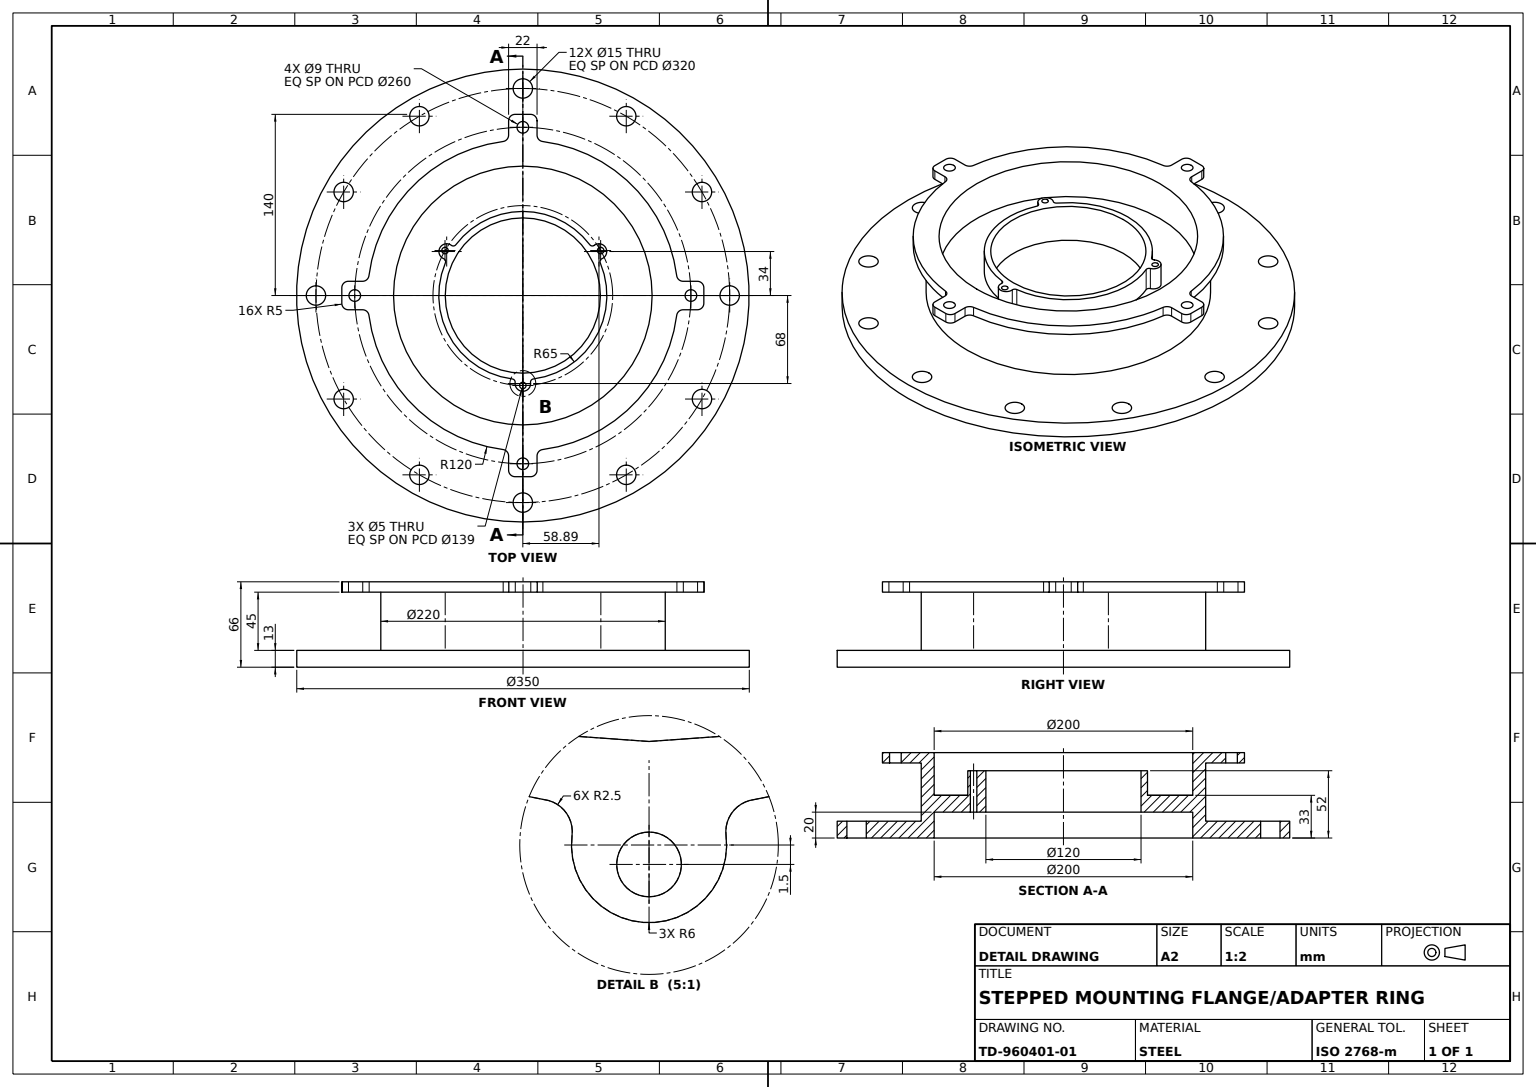
from build123d import *

# Parameters (mm, degrees)
BASE_FLANGE_SKETCH_R      = 175
BASE_FLANGE_350_DEPTH     = 13
HUB_SKETCH_R              = 110
HUB_BOSS_220_DEPTH        = 45
MOUNTING_LUGS_4X_DEPTH    = 8
BOLT_HOLES_SKETCH_R       = 7.5
BOLT_HOLES_12X_15_DEPTH   = 111
UPPER_BORE_SKETCH_R       = 100
UPPER_BORE_200_DEPTH      = 20
INNER_RECESS_SKETCH_R     = 33
INNER_RECESS_CUT_DEPTH    = 13
LOWER_BORE_SKETCH_R       = 100
LOWER_BORE_200_DEPTH      = 53
INNER_RING_BOSS_DEPTH     = 32
CENTRE_BORE_SKETCH_R      = 60
CENTRE_BORE_120_DEPTH     = 62
LUG_NOTCH_SKETCH_R        = 4.5
LUG_NOTCH_CUT_DEPTH       = 48
INNER_RING_SLOTS_SKETCH_R = 2.5
INNER_RING_SLOTS_3X_DEPTH = 48


with BuildPart() as part:
    # Base Flange Sketch → Base Flange Ø350 (new body)
    with BuildSketch(Plane(origin=(0, 0, 0), x_dir=(1, 0, 0), z_dir=(0, 1, 0))):
        with Locations(Location((0, 0, 0), (0, 0, 90))):
            Circle(BASE_FLANGE_SKETCH_R)
    extrude(amount=BASE_FLANGE_350_DEPTH)

    # Hub Sketch → Hub Boss Ø220 (add)
    with BuildSketch(Plane(origin=(0, 13, 0), x_dir=(1, 0, 0), z_dir=(0, 1, 0))):
        with Locations(Location((0, 0, 0), (0, 0, 90))):
            Circle(HUB_SKETCH_R)
    extrude(amount=HUB_BOSS_220_DEPTH)

    # Mounting Lugs Sketch → Mounting Lugs 4x (add)
    with BuildSketch(Plane(origin=(0, 58, 0), x_dir=(1, 0, 0), z_dir=(0, 1, 0))):
        with BuildLine():
            Line((123.97177098, 11), (135, 11))
            ThreePointArc((135, 11), (138.535533906, 9.535533906), (140, 6))
            Line((140, 6), (140, 0))
            Line((140, 0), (140, -6.000000959))
            ThreePointArc((140, -6.000000959), (138.535533906, -9.535534865), (135, -11.000000959))
            Line((135, -11.000000959), (123.971770857, -11.000000959))
            ThreePointArc((123.971770857, -11.000000959), (120.670256067, -12.245004275), (119.012900022, -15.360000921))
            ThreePointArc((119.012900022, -15.360000921), (84.852813414, -84.852814071), (15.36, -119.012900141))
            ThreePointArc((15.36, -119.012900141), (12.245003329, -120.670256176), (11, -123.97177098))
            Line((11, -123.97177098), (11, -135))
            ThreePointArc((11, -135), (9.535533906, -138.535533906), (6, -140))
            Line((6, -140), (0, -140))
            Line((0, -140), (-6.000000959, -140))
            ThreePointArc((-6.000000959, -140), (-9.535534865, -138.535533906), (-11.000000959, -135))
            Line((-11.000000959, -135), (-11.000000959, -123.971770857))
            ThreePointArc((-11.000000959, -123.971770857), (-12.245004275, -120.670256067), (-15.360000921, -119.012900022))
            ThreePointArc((-15.360000921, -119.012900022), (-84.852814071, -84.852813414), (-119.012900141, -15.36))
            ThreePointArc((-119.012900141, -15.36), (-120.670256176, -12.245003329), (-123.97177098, -11))
            Line((-123.97177098, -11), (-135, -11))
            ThreePointArc((-135, -11), (-138.535533906, -9.535533906), (-140, -6))
            Line((-140, -6), (-140, 0))
            Line((-140, 0), (-140, 6.000000959))
            ThreePointArc((-140, 6.000000959), (-138.535533906, 9.535534865), (-135, 11.000000959))
            Line((-135, 11.000000959), (-123.971770857, 11.000000959))
            ThreePointArc((-123.971770857, 11.000000959), (-120.670256067, 12.245004275), (-119.012900022, 15.360000921))
            ThreePointArc((-119.012900022, 15.360000921), (-84.852813414, 84.852814071), (-15.36, 119.012900141))
            ThreePointArc((-15.36, 119.012900141), (-12.245003329, 120.670256176), (-11, 123.97177098))
            Line((-11, 123.97177098), (-11, 135))
            ThreePointArc((-11, 135), (-9.535533906, 138.535533906), (-6, 140))
            Line((-6, 140), (0, 140))
            Line((0, 140), (6.000000959, 140))
            ThreePointArc((6.000000959, 140), (9.535534865, 138.535533906), (11.000000959, 135))
            Line((11.000000959, 135), (11.000000959, 123.971770857))
            ThreePointArc((11.000000959, 123.971770857), (12.245004275, 120.670256067), (15.360000921, 119.012900022))
            ThreePointArc((15.360000921, 119.012900022), (84.852814071, 84.852813414), (119.012900141, 15.36))
            ThreePointArc((119.012900141, 15.36), (120.670256176, 12.245003329), (123.97177098, 11))
        make_face()
    extrude(amount=MOUNTING_LUGS_4X_DEPTH)

    # Bolt Holes Sketch → Bolt Holes 12xØ15 (cut)
    with BuildSketch(Plane(origin=(0, 13, 0), x_dir=(1, 0, 0), z_dir=(0, 1, 0))):
        with Locations(Location((0, 160, 0), (0, 0, 270))):
            Circle(BOLT_HOLES_SKETCH_R)
        with Locations(Location((80, 138.564064606, 0), (0, 0, 270))):
            Circle(BOLT_HOLES_SKETCH_R)
        with Locations(Location((138.564064606, 80, 0), (0, 0, 270))):
            Circle(BOLT_HOLES_SKETCH_R)
        with Locations(Location((160, 0, 0), (0, 0, 270))):
            Circle(BOLT_HOLES_SKETCH_R)
        with Locations(Location((138.564064606, -80, 0), (0, 0, 270))):
            Circle(BOLT_HOLES_SKETCH_R)
        with Locations(Location((80, -138.564064605, 0), (0, 0, 270))):
            Circle(BOLT_HOLES_SKETCH_R)
        with Locations(Location((0, -160, 0), (0, 0, 270))):
            Circle(BOLT_HOLES_SKETCH_R)
        with Locations(Location((-80, -138.564064606, 0), (0, 0, 270))):
            Circle(BOLT_HOLES_SKETCH_R)
        with Locations(Location((-138.564064605, -80, 0), (0, 0, 270))):
            Circle(BOLT_HOLES_SKETCH_R)
        with Locations(Location((-160, 0, 0), (0, 0, 270))):
            Circle(BOLT_HOLES_SKETCH_R)
        with Locations(Location((-138.564064605, 80, 0), (0, 0, 270))):
            Circle(BOLT_HOLES_SKETCH_R)
        with Locations(Location((-80, 138.564064605, 0), (0, 0, 270))):
            Circle(BOLT_HOLES_SKETCH_R)
    extrude(amount=-BOLT_HOLES_12X_15_DEPTH, mode=Mode.SUBTRACT)

    # Upper Bore Sketch → Upper Bore Ø200 (cut)
    with BuildSketch(Plane.XZ):
        with Locations(Location((0, 0, 0), (0, 0, 270))):
            Circle(UPPER_BORE_SKETCH_R)
    extrude(amount=-UPPER_BORE_200_DEPTH, mode=Mode.SUBTRACT)

    # Inner Recess Sketch → Inner Recess Cut (cut)
    with BuildSketch(Plane.XZ.offset(-20)):
        with Locations(Location((0, 0, 0), (0, 0, 270))):
            Circle(INNER_RECESS_SKETCH_R)
    extrude(amount=-INNER_RECESS_CUT_DEPTH, mode=Mode.SUBTRACT)

    # Lower Bore Sketch → Lower Bore Ø200 (cut)
    with BuildSketch(Plane.XZ.offset(-33)):
        with Locations(Location((0, 0, 0), (0, 0, 270))):
            Circle(LOWER_BORE_SKETCH_R)
    extrude(amount=-LOWER_BORE_200_DEPTH, mode=Mode.SUBTRACT)

    # Inner Ring Sketch → Inner Ring Boss (add)
    with BuildSketch(Plane.XZ.offset(-20)):
        with BuildLine():
            ThreePointArc((-8.124937524, 64.490196078), (-56.291651246, 32.5), (-59.912616861, -25.208695739))
            ThreePointArc((-59.912616861, -25.208695739), (-59.900107579, -27.117542161), (-61.238353919, -28.478772442))
            ThreePointArc((-61.238353919, -28.478772442), (-64.08587988, -37), (-55.282517363, -38.794583959))
            ThreePointArc((-55.282517363, -38.794583959), (-53.43453419, -38.316243773), (-51.787679337, -39.281500339))
            ThreePointArc((-51.787679337, -39.281500339), (0, -65), (51.787679337, -39.281500339))
            ThreePointArc((51.787679337, -39.281500339), (53.43453419, -38.316243773), (55.282517363, -38.794583959))
            ThreePointArc((55.282517363, -38.794583959), (64.08587988, -37), (61.238353919, -28.478772442))
            ThreePointArc((61.238353919, -28.478772442), (59.900107579, -27.117542161), (59.912616861, -25.208695739))
            ThreePointArc((59.912616861, -25.208695739), (56.291651246, 32.5), (8.124937524, 64.490196078))
            ThreePointArc((8.124937524, 64.490196078), (6.46557339, 65.433785934), (5.955836556, 67.273356401))
            ThreePointArc((5.955836556, 67.273356401), (0, 74), (-5.955836556, 67.273356401))
            ThreePointArc((-5.955836556, 67.273356401), (-6.46557339, 65.433785934), (-8.124937524, 64.490196078))
        make_face()
    extrude(amount=-INNER_RING_BOSS_DEPTH)

    # Centre Bore Sketch → Centre Bore Ø120 (cut)
    with BuildSketch(Plane(origin=(0, 52, 0), x_dir=(1, 0, 0), z_dir=(0, 1, 0))):
        with Locations(Location((0, 0, 0), (0, 0, 270))):
            Circle(CENTRE_BORE_SKETCH_R)
    extrude(amount=-CENTRE_BORE_120_DEPTH, mode=Mode.SUBTRACT)

    # Lug Notch Sketch → Lug Notch Cut (cut)
    with BuildSketch(Plane(origin=(0, 66, 0), x_dir=(1, 0, 0), z_dir=(0, 1, 0))):
        with Locations(Location((0, 130, 0), (0, 0, 270))):
            Circle(LUG_NOTCH_SKETCH_R)
        with Locations(Location((130, 0, 0), (0, 0, 270))):
            Circle(LUG_NOTCH_SKETCH_R)
        with Locations(Location((0, -130, 0), (0, 0, 270))):
            Circle(LUG_NOTCH_SKETCH_R)
        with Locations(Location((-130, 0, 0), (0, 0, 270))):
            Circle(LUG_NOTCH_SKETCH_R)
    extrude(amount=-LUG_NOTCH_CUT_DEPTH, mode=Mode.SUBTRACT)

    # Inner Ring Slots Sketch → Inner Ring Slots 3x (cut)
    with BuildSketch(Plane(origin=(0, 52, 0), x_dir=(1, 0, 0), z_dir=(0, 1, 0))):
        with Locations(Location((0, -69.5, 0), (0, 0, 270))):
            Circle(INNER_RING_SLOTS_SKETCH_R)
        with Locations(Location((-60.188765563, 34.75, 0), (0, 0, 270))):
            Circle(INNER_RING_SLOTS_SKETCH_R)
        with Locations(Location((60.188765563, 34.75, 0), (0, 0, 270))):
            Circle(INNER_RING_SLOTS_SKETCH_R)
    extrude(amount=-INNER_RING_SLOTS_3X_DEPTH, mode=Mode.SUBTRACT)


solid = part.part
